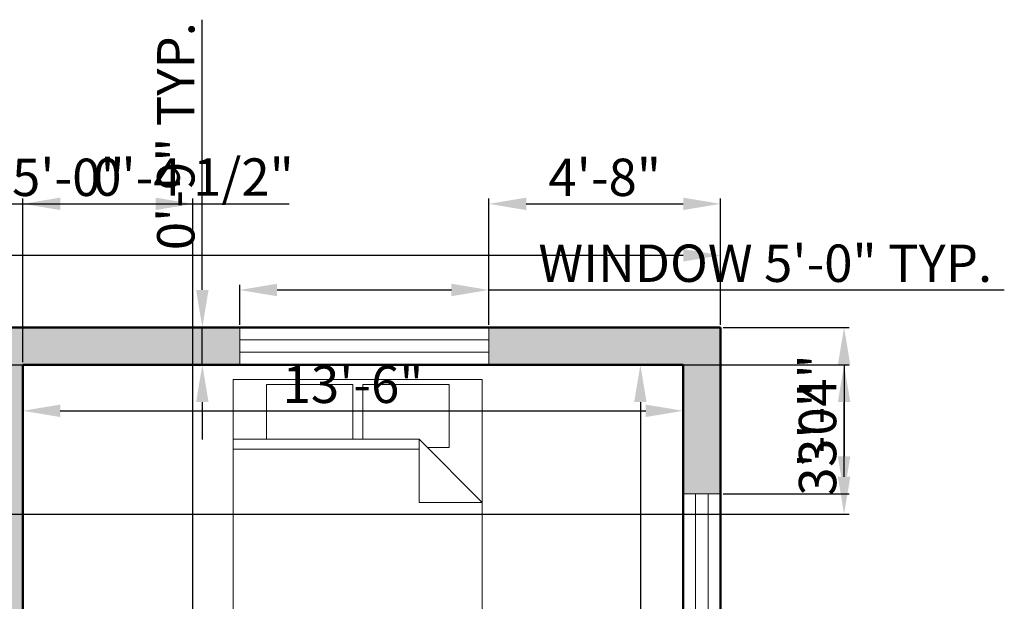
# Model space of a CAD drawing. Units: inches. Extents: x 875413 to 876020, y 447446 to 448210.
# Tile 8 of 8: x 875767 to 876004, y 448013 to 448153. Entities that reach past the tile are written whole.
import ezdxf

# ---------------------------------------------------------------- set-up
doc = ezdxf.new("R2010")
doc.units = ezdxf.units.IN
for name, color, linetype, lineweight in [('A-ANNO-DIMS', 2, 'Continuous', 13), ('A-FURN', 8, 'Continuous', 18), ('A-GLAZ', 4, 'Continuous', 20), ('A-WALL', 7, 'Continuous', 50)]:
    doc.layers.add(name, color=color, linetype=linetype, lineweight=lineweight)
doc.layers.add('A-WALL-PATT', color=18, linetype='Continuous', lineweight=13, true_color=0x000000)
doc.styles.get("Standard").update_dxf_attribs({"font": 'arial.ttf'})
doc.dimstyles.new('ISO-25', dxfattribs={"dimtxt": 9, "dimasz": 9, "dimexe": 1.25, "dimexo": 0.625, "dimtad": 1, "dimdec": 1, "dimrnd": 9, "dimlunit": 3, "dimtxsty": 'Standard', "dimcen": 2.5, "dimadec": 0, "dimazin": 0, "dimtfac": 1, "dimtdec": 1, "dimtmove": 0, "dimatfit": 3, "dimfxl": 1, "dimarcsym": 0})

# ---------------------------------------------------------------- blocks, each defined once
blk = doc.blocks.new('*D5')
at = {"layer": 'A-ANNO-DIMS', "color": 0, "lineweight": -2, "transparency": 16777216}
for p, q in [((875767.7, 448069.39), (875767.7, 448057.67)), ((875926.7, 448069.39), (875926.7, 448057.67)), ((875776.7, 448058.92), (875917.7, 448058.92))]:
    blk.add_line(p, q, dxfattribs=at)
at = {"layer": 'A-ANNO-DIMS', "color": 0, "transparency": 16777216}
for points in [[(875776.7, 448060.42), (875776.7, 448057.42), (875767.7, 448058.92)], [(875917.7, 448060.42), (875917.7, 448057.42), (875926.7, 448058.92)]]:
    blk.add_solid(points, dxfattribs=at)
at = {"layer": 'Defpoints', "color": 0, "transparency": 16777216}
for p in [(875767.7, 448070.02), (875926.7, 448070.02), (875926.7, 448058.92)]:
    blk.add_point(p, dxfattribs=at)
at = {"layer": 'A-ANNO-DIMS', "color": 0, "transparency": 16777216, "insert": (875847.2, 448064.14), "char_height": 9, "attachment_point": 5}
blk.add_mtext('13\'-6"', dxfattribs=at)
blk = doc.blocks.new('*D6')
at = {"layer": 'A-ANNO-DIMS', "color": 0, "lineweight": -2, "transparency": 16777216}
for p, q in [((875926.08, 448070.02), (875915.14, 448070.02)), ((875916.39, 448061.02), (875916.39, 447930.52)), ((875926.08, 447921.52), (875915.14, 447921.52))]:
    blk.add_line(p, q, dxfattribs=at)
at = {"layer": 'A-ANNO-DIMS', "color": 0, "transparency": 16777216}
for points in [[(875914.89, 448061.02), (875917.89, 448061.02), (875916.39, 448070.02)], [(875914.89, 447930.52), (875917.89, 447930.52), (875916.39, 447921.52)]]:
    blk.add_solid(points, dxfattribs=at)
at = {"layer": 'Defpoints', "color": 0, "transparency": 16777216}
for p in [(875926.7, 448070.02), (875916.39, 447921.52), (875926.7, 447921.52)]:
    blk.add_point(p, dxfattribs=at)
at = {"layer": 'A-ANNO-DIMS', "color": 0, "transparency": 16777216, "insert": (875911.25, 447995.77), "char_height": 9, "attachment_point": 5, "rotation": 90}
blk.add_mtext("12'", dxfattribs=at)
blk = doc.blocks.new('Bed - Queen')
for p, q in [((0, -80.00003), (0, 0)), ((0, 0), (59.99999, 0)), ((59.99999, 0), (59.99999, -80.00003)), ((7.99999, -1.2), (28.79998, -1.2)), ((7.99999, -14.4), (7.99999, -1.2)), ((28.79998, -1.2), (28.79998, -14.4)), ((31.19999, -1.2), (51.99999, -1.2)), ((31.19999, -14.4), (31.19999, -1.2)), ((51.99999, -1.2), (51.99999, -16.4)), ((0, -14.4), (44.8, -14.4)), ((59.99999, -29.6), (44.8, -14.4)), ((44.8, -14.4), (44.8, -29.6)), ((51.99999, -16.4), (46.79936, -16.4)), ((44.8, -16.8), (0, -16.8)), ((44.8, -29.6), (59.99999, -29.6)), ((59.99999, -80.00003), (0, -80.00003))]:
    blk.add_line(p, q)
blk = doc.blocks.new('*D37')
at = {"layer": 'A-ANNO-DIMS', "color": 0, "lineweight": -2, "transparency": 16777216}
for p, q in [((875461.7, 448079.64), (875461.7, 448097.63)), ((875935.7, 448079.64), (875935.7, 448097.63)), ((875470.7, 448096.38), (875926.7, 448096.38))]:
    blk.add_line(p, q, dxfattribs=at)
at = {"layer": 'A-ANNO-DIMS', "color": 0, "transparency": 16777216}
for points in [[(875470.7, 448097.88), (875470.7, 448094.88), (875461.7, 448096.38)], [(875926.7, 448097.88), (875926.7, 448094.88), (875935.7, 448096.38)]]:
    blk.add_solid(points, dxfattribs=at)
at = {"layer": 'Defpoints', "color": 0, "transparency": 16777216}
for p in [(875935.7, 448096.38), (875461.7, 448079.02), (875935.7, 448079.02)]:
    blk.add_point(p, dxfattribs=at)
at = {"layer": 'A-ANNO-DIMS', "color": 0, "transparency": 16777216, "insert": (875698.7, 448101.6), "char_height": 9, "attachment_point": 5}
blk.add_mtext('39\'-9"', dxfattribs=at)
blk = doc.blocks.new('WIN-60IN')
for p, q in [((0, 9), (0, 0)), ((60, 9), (60, 0)), ((60, 6), (0, 6)), ((60, 3), (0, 3))]:
    blk.add_line(p, q)
blk = doc.blocks.new('*D41')
at = {"layer": 'A-ANNO-DIMS', "color": 0, "lineweight": -2, "transparency": 16777216}
for p, q in [((875819.9, 448079.64), (875819.9, 448089.27)), ((875828.9, 448088.02), (875870.9, 448088.02)), ((875879.9, 448079.64), (875879.9, 448089.27)), ((875879.9, 448088.02), (876004.04, 448088.02))]:
    blk.add_line(p, q, dxfattribs=at)
at = {"layer": 'A-ANNO-DIMS', "color": 0, "transparency": 16777216}
for points in [[(875828.9, 448089.52), (875828.9, 448086.52), (875819.9, 448088.02)], [(875870.9, 448089.52), (875870.9, 448086.52), (875879.9, 448088.02)]]:
    blk.add_solid(points, dxfattribs=at)
at = {"layer": 'Defpoints', "color": 0, "transparency": 16777216}
for p in [(875879.9, 448088.02), (875819.9, 448079.02), (875879.9, 448079.02)]:
    blk.add_point(p, dxfattribs=at)
at = {"layer": 'A-ANNO-DIMS', "color": 0, "transparency": 16777216, "insert": (875946.47, 448093.3), "char_height": 9, "attachment_point": 5}
blk.add_mtext('WINDOW 5\'-0" TYP.', dxfattribs=at)
blk = doc.blocks.new('*D42')
at = {"layer": 'A-ANNO-DIMS', "color": 0, "lineweight": -2, "transparency": 16777216}
for p, q in [((875810.9, 448088.02), (875810.9, 448153.13)), ((875819.27, 448079.02), (875809.65, 448079.02)), ((875810.9, 448070.02), (875810.9, 448079.02)), ((875819.27, 448070.02), (875809.65, 448070.02)), ((875810.9, 448061.02), (875810.9, 448052.02))]:
    blk.add_line(p, q, dxfattribs=at)
at = {"layer": 'A-ANNO-DIMS', "color": 0, "transparency": 16777216}
for points in [[(875809.4, 448088.02), (875812.4, 448088.02), (875810.9, 448079.02)], [(875809.4, 448061.02), (875812.4, 448061.02), (875810.9, 448070.02)]]:
    blk.add_solid(points, dxfattribs=at)
at = {"layer": 'Defpoints', "color": 0, "transparency": 16777216}
for p in [(875810.9, 448079.02), (875819.9, 448079.02), (875819.9, 448070.02)]:
    blk.add_point(p, dxfattribs=at)
at = {"layer": 'A-ANNO-DIMS', "color": 0, "transparency": 16777216, "insert": (875805.68, 448125.07), "char_height": 9, "attachment_point": 5, "rotation": 90}
blk.add_mtext('0\'-9" TYP.', dxfattribs=at)
blk = doc.blocks.new('*D68')
at = {"layer": 'A-ANNO-DIMS', "color": 0, "lineweight": -2, "transparency": 16777216}
for p, q in [((875879.9, 448079.64), (875879.9, 448110.02)), ((875888.9, 448108.77), (875926.7, 448108.77)), ((875935.7, 448079.64), (875935.7, 448110.02))]:
    blk.add_line(p, q, dxfattribs=at)
at = {"layer": 'A-ANNO-DIMS', "color": 0, "transparency": 16777216}
for points in [[(875888.9, 448110.27), (875888.9, 448107.27), (875879.9, 448108.77)], [(875926.7, 448110.27), (875926.7, 448107.27), (875935.7, 448108.77)]]:
    blk.add_solid(points, dxfattribs=at)
at = {"layer": 'Defpoints', "color": 0, "transparency": 16777216}
for p in [(875935.7, 448108.77), (875879.9, 448079.02), (875935.7, 448079.02)]:
    blk.add_point(p, dxfattribs=at)
at = {"layer": 'A-ANNO-DIMS', "color": 0, "transparency": 16777216, "insert": (875907.8, 448113.99), "char_height": 9, "attachment_point": 5}
blk.add_mtext('4\'-8"', dxfattribs=at)
blk = doc.blocks.new('*D70')
at = {"layer": 'A-ANNO-DIMS', "color": 0, "lineweight": -2, "transparency": 16777216}
for p, q in [((875936.33, 448079.02), (875966.7, 448079.02)), ((875965.45, 448070.02), (875965.45, 448047.92)), ((875936.33, 448038.92), (875966.7, 448038.92))]:
    blk.add_line(p, q, dxfattribs=at)
at = {"layer": 'A-ANNO-DIMS', "color": 0, "transparency": 16777216}
for points in [[(875963.95, 448070.02), (875966.95, 448070.02), (875965.45, 448079.02)], [(875963.95, 448047.92), (875966.95, 448047.92), (875965.45, 448038.92)]]:
    blk.add_solid(points, dxfattribs=at)
at = {"layer": 'Defpoints', "color": 0, "transparency": 16777216}
for p in [(875935.7, 448079.02), (875935.7, 448038.92), (875965.45, 448038.92)]:
    blk.add_point(p, dxfattribs=at)
at = {"layer": 'A-ANNO-DIMS', "color": 0, "transparency": 16777216, "insert": (875960.23, 448058.97), "char_height": 9, "attachment_point": 5, "rotation": 90}
blk.add_mtext('3\'-4"', dxfattribs=at)
blk = doc.blocks.new('*D80')
at = {"layer": 'A-ANNO-DIMS', "color": 0, "lineweight": -2, "transparency": 16777216}
for p, q in [((875748.63, 447673.14), (875748.63, 448110.02)), ((875757.63, 448108.77), (875799.63, 448108.77)), ((875808.63, 447673.14), (875808.63, 448110.02))]:
    blk.add_line(p, q, dxfattribs=at)
at = {"layer": 'A-ANNO-DIMS', "color": 0, "transparency": 16777216}
for points in [[(875757.63, 448110.27), (875757.63, 448107.27), (875748.63, 448108.77)], [(875799.63, 448110.27), (875799.63, 448107.27), (875808.63, 448108.77)]]:
    blk.add_solid(points, dxfattribs=at)
at = {"layer": 'Defpoints', "color": 0, "transparency": 16777216}
for p in [(875808.63, 448108.77), (875748.63, 447672.52), (875808.63, 447672.52)]:
    blk.add_point(p, dxfattribs=at)
at = {"layer": 'A-ANNO-DIMS', "color": 0, "transparency": 16777216, "insert": (875778.63, 448113.99), "char_height": 9, "attachment_point": 5}
blk.add_mtext('5\'-0"', dxfattribs=at)
blk = doc.blocks.new('*D81')
at = {"layer": 'A-ANNO-DIMS', "color": 0, "lineweight": -2, "transparency": 16777216}
for p, q in [((875754.2, 448108.77), (875745.2, 448108.77)), ((875763.2, 448070.64), (875763.2, 448110.02)), ((875763.2, 448108.77), (875767.7, 448108.77)), ((875767.7, 448070.64), (875767.7, 448110.02)), ((875776.7, 448108.77), (875831.85, 448108.77))]:
    blk.add_line(p, q, dxfattribs=at)
at = {"layer": 'A-ANNO-DIMS', "color": 0, "transparency": 16777216}
for points in [[(875754.2, 448110.27), (875754.2, 448107.27), (875763.2, 448108.77)], [(875776.7, 448110.27), (875776.7, 448107.27), (875767.7, 448108.77)]]:
    blk.add_solid(points, dxfattribs=at)
at = {"layer": 'Defpoints', "color": 0, "transparency": 16777216}
for p in [(875767.7, 448108.77), (875763.2, 448070.02), (875767.7, 448070.02)]:
    blk.add_point(p, dxfattribs=at)
at = {"layer": 'A-ANNO-DIMS', "color": 0, "transparency": 16777216, "insert": (875808.78, 448114.05), "char_height": 9, "attachment_point": 5}
blk.add_mtext('0\'-4 1/2"', dxfattribs=at)
blk = doc.blocks.new('*D87')
at = {"layer": 'A-ANNO-DIMS', "color": 0, "lineweight": -2, "transparency": 16777216}
for p, q in [((875763.83, 448070.02), (875966.7, 448070.02)), ((875965.45, 448043.02), (875965.45, 448061.02)), ((875763.83, 448034.02), (875966.7, 448034.02))]:
    blk.add_line(p, q, dxfattribs=at)
at = {"layer": 'A-ANNO-DIMS', "color": 0, "transparency": 16777216}
for points in [[(875963.95, 448061.02), (875966.95, 448061.02), (875965.45, 448070.02)], [(875963.95, 448043.02), (875966.95, 448043.02), (875965.45, 448034.02)]]:
    blk.add_solid(points, dxfattribs=at)
at = {"layer": 'Defpoints', "color": 0, "transparency": 16777216}
for p in [(875763.2, 448070.02), (875965.45, 448070.02), (875763.2, 448034.02)]:
    blk.add_point(p, dxfattribs=at)
at = {"layer": 'A-ANNO-DIMS', "color": 0, "transparency": 16777216, "insert": (875960.23, 448052.02), "char_height": 9, "attachment_point": 5, "rotation": 90}
blk.add_mtext('3\'-0"', dxfattribs=at)

msp = doc.modelspace()

# ---------------------------------------------------------------- hatches: boundary and pattern name
at = {"layer": 'A-WALL-PATT'}
h = msp.add_hatch(color=256, dxfattribs=at)
h.dxf.hatch_style = 1
h.paths.add_polyline_path([(875470.7, 447985.13), (875461.7, 447985.13), (875461.7, 447865.29), (875470.7, 447865.29), (875470.7, 447881.02), (875566.7, 447881.02), (875566.7, 447797.02), (875571.2, 447797.02), (875571.2, 447885.52), (875571.2, 447921.52), (875603.29, 447921.52), (875603.29, 447926.02), (875501.27, 447926.02), (875501.27, 447921.52), (875566.7, 447921.52), (875566.7, 447885.52), (875470.7, 447885.52), (875470.7, 447921.52), (875470.7, 447926.02)])
h.paths.add_polyline_path([(875470.7, 448070.02), (875518.96, 448070.02), (875518.96, 448079.02), (875461.7, 448079.02), (875461.7, 448045.13), (875470.7, 448045.13)])
h.paths.add_polyline_path([(875819.9, 448079.02), (875578.96, 448079.02), (875578.96, 448070.02), (875638.7, 448070.02), (875638.7, 447921.52), (875643.2, 447921.52), (875643.2, 448070.02), (875763.2, 448070.02), (875763.2, 447921.52), (875767.7, 447921.52), (875767.7, 448070.02), (875819.9, 448070.02)])
h.paths.add_polyline_path([(875935.7, 447978.92), (875926.7, 447978.92), (875926.7, 447926.02), (875926.7, 447921.52), (875926.7, 447885.52), (875842.7, 447885.52), (875842.7, 447921.52), (875899.7, 447921.52), (875899.7, 447926.02), (875805.34, 447926.02), (875805.34, 447921.52), (875838.2, 447921.52), (875838.2, 447885.52), (875838.2, 447797.02), (875689.7, 447797.02), (875689.7, 447792.52), (875842.7, 447792.52), (875842.7, 447881.02), (875926.7, 447881.02), (875926.7, 447857.16), (875935.7, 447857.16)])
h.paths.add_polyline_path([(875935.7, 448079.02), (875879.9, 448079.02), (875879.9, 448070.02), (875926.7, 448070.02), (875926.7, 448038.92), (875935.7, 448038.92)])
h.paths.add_polyline_path([(875935.7, 447833.16), (875926.7, 447833.16), (875926.7, 447797.02), (875842.7, 447797.02), (875842.7, 447792.52), (875926.7, 447792.52), (875926.7, 447756.52), (875935.7, 447756.52)])
h.paths.add_polyline_path([(875935.7, 447732.52), (875926.7, 447732.52), (875926.7, 447692.75, -0.007222), (875926.81, 447692.41, -0.08192), (875927.45, 447687.6, -0.071798), (875926.7, 447683.4), (875926.7, 447672.52), (875808.63, 447672.52), (875808.63, 447668.02), (875926.7, 447668.02), (875926.7, 447663.19), (875935.7, 447663.19)])
h.paths.add_polyline_path([(875842.7, 447792.52), (875838.2, 447792.52), (875838.2, 447704.02), (875842.7, 447704.02)])
h.paths.add_polyline_path([(875470.7, 447792.52), (875619.2, 447792.52), (875619.2, 447797.02), (875470.7, 447797.02), (875470.7, 447841.29), (875461.7, 447841.29), (875461.7, 447764.71), (875470.7, 447764.71)])
h.paths.add_polyline_path([(875619.2, 447760.51), (875616.95, 447760.51, -0.018388), (875614.7, 447760.37), (875614.7, 447672.52), (875470.7, 447672.52), (875470.7, 447704.71), (875461.7, 447704.71), (875461.7, 447640.7), (875470.7, 447640.7), (875470.7, 447668.02), (875619.2, 447668.02)])
h.paths.add_polyline_path([(875511.12, 447554.02), (875470.7, 447554.02), (875470.7, 447580.7), (875461.7, 447580.7), (875461.7, 447545.02), (875511.12, 447545.02)])
h.paths.add_polyline_path([(875656.47, 447554.02), (875620.05, 447554.02, -0.057036), (875616.67, 447553.74, -0.040891), (875614.26, 447554.02), (875571.12, 447554.02), (875571.12, 447545.02), (875656.47, 447545.02)])
h.paths.add_polyline_path([(875643.2, 447613.27), (875685.21, 447613.27), (875685.21, 447617.77), (875685.21, 447623.8), (875680.71, 447623.8), (875680.71, 447617.77), (875618.23, 447617.77), (875618.23, 447623.8), (875613.73, 447623.8), (875613.73, 447617.77), (875613.73, 447613.27), (875638.7, 447613.27), (875638.7, 447554.02), (875643.2, 447554.02)])
h.paths.add_polyline_path([(875694.2, 447760.28), (875689.7, 447760.28), (875689.7, 447668.02), (875748.63, 447668.02), (875748.63, 447672.52), (875694.2, 447672.52)])

# ---------------------------------------------------------------- linework, layer by layer
at = {"layer": 'A-WALL'}
for p, q in [((875935.7, 448079.02), (875461.7, 448079.02)), ((875935.7, 447663.19), (875935.7, 448079.02)), ((875926.7, 448070.02), (875767.7, 448070.02)), ((875767.7, 448070.02), (875767.7, 447921.52)), ((875926.7, 447926.02), (875926.7, 448070.02))]:
    msp.add_line(p, q, dxfattribs=at)

# ---------------------------------------------------------------- block references
at = {"layer": 'A-FURN'}
msp.add_blockref('Bed - Queen', (875818.33, 448066.46), dxfattribs=at)
at = {"layer": 'A-GLAZ'}
msp.add_blockref('WIN-60IN', (875819.9, 448070.02), dxfattribs=at)
at = {"layer": 'A-GLAZ', "rotation": 269.9999999998151}
msp.add_blockref('WIN-60IN', (875926.7, 448038.92), dxfattribs=at)

# ---------------------------------------------------------------- dimensions: what is measured, and where the dimension line sits
at = {"layer": 'A-ANNO-DIMS'}
dim = msp.add_linear_dim(base=(875810.9, 448079.02), p1=(875819.9, 448070.02), p2=(875819.9, 448079.02), angle=90, text='<> TYP.', dimstyle='ISO-25', override={"dimdec": 1, "dimlfac": 1, "dimrnd": 0, "dimzin": 1, "dimdsep": 46, "dimlunit": 4, "dimfrac": 2}, dxfattribs=at)
dim.commit()
dim.dimension.update_dxf_attribs({"geometry": '*D42', "text_midpoint": (875805.68, 448125.07)})
for base, p1, p2, override, picture, middle in [((875767.7, 448108.77), (875763.2, 448070.02), (875767.7, 448070.02), {"dimdec": 1, "dimlfac": 1, "dimrnd": 0, "dimzin": 1, "dimdsep": 46, "dimlunit": 4, "dimfrac": 2}, '*D81', (875808.78, 448114.05)), ((875808.63, 448108.77), (875748.63, 447672.52), (875808.63, 447672.52), {"dimdec": 1, "dimlfac": 1, "dimrnd": 0, "dimzin": 1, "dimdsep": 46, "dimlunit": 4, "dimfrac": 2}, '*D80', (875778.63, 448113.99)), ((875935.7, 448108.77), (875879.9, 448079.02), (875935.7, 448079.02), {"dimdec": 1, "dimlfac": 1, "dimrnd": 0, "dimzin": 1, "dimdsep": 46, "dimlunit": 4, "dimfrac": 2}, '*D68', (875907.8, 448113.99)), ((875935.7, 448096.38), (875461.7, 448079.02), (875935.7, 448079.02), {"dimclrd": 0, "dimclre": 0, "dimclrt": 0}, '*D37', (875698.7, 448101.6)), ((875926.7, 448058.92), (875767.7, 448070.02), (875926.7, 448070.02), {"dimclrd": 0, "dimclre": 0, "dimclrt": 0}, '*D5', (875847.2, 448064.14))]:
    dim = msp.add_linear_dim(base=base, p1=p1, p2=p2, dimstyle='ISO-25', override=override, dxfattribs=at)
    dim.commit()
    dim.dimension.update_dxf_attribs({"geometry": picture, "text_midpoint": middle})
dim = msp.add_linear_dim(base=(875879.9, 448088.02), p1=(875819.9, 448079.02), p2=(875879.9, 448079.02), text='WINDOW <> TYP.', dimstyle='ISO-25', override={"dimdec": 1, "dimlfac": 1, "dimrnd": 0, "dimzin": 1, "dimdsep": 46, "dimlunit": 4, "dimfrac": 2}, dxfattribs=at)
dim.commit()
dim.dimension.update_dxf_attribs({"geometry": '*D41', "text_midpoint": (875946.47, 448093.3)})
for base, p1, p2, override, picture, middle in [((875965.45, 448038.92), (875935.7, 448079.02), (875935.7, 448038.92), {"dimdec": 1, "dimlfac": 1, "dimrnd": 0, "dimzin": 1, "dimdsep": 46, "dimlunit": 4, "dimfrac": 2}, '*D70', (875960.23, 448058.97)), ((875965.45, 448070.02), (875763.2, 448034.02), (875763.2, 448070.02), {"dimdec": 1, "dimlfac": 1, "dimrnd": 0, "dimzin": 1, "dimdsep": 46, "dimlunit": 4, "dimfrac": 2}, '*D87', (875960.23, 448052.02)), ((875916.39, 447921.52), (875926.7, 448070.02), (875926.7, 447921.52), {"dimclrd": 0, "dimclre": 0, "dimclrt": 0}, '*D6', (875911.25, 447995.77))]:
    dim = msp.add_linear_dim(base=base, p1=p1, p2=p2, angle=90, dimstyle='ISO-25', override=override, dxfattribs=at)
    dim.commit()
    dim.dimension.update_dxf_attribs({"geometry": picture, "text_midpoint": middle})

doc.saveas('drawing.dxf')
